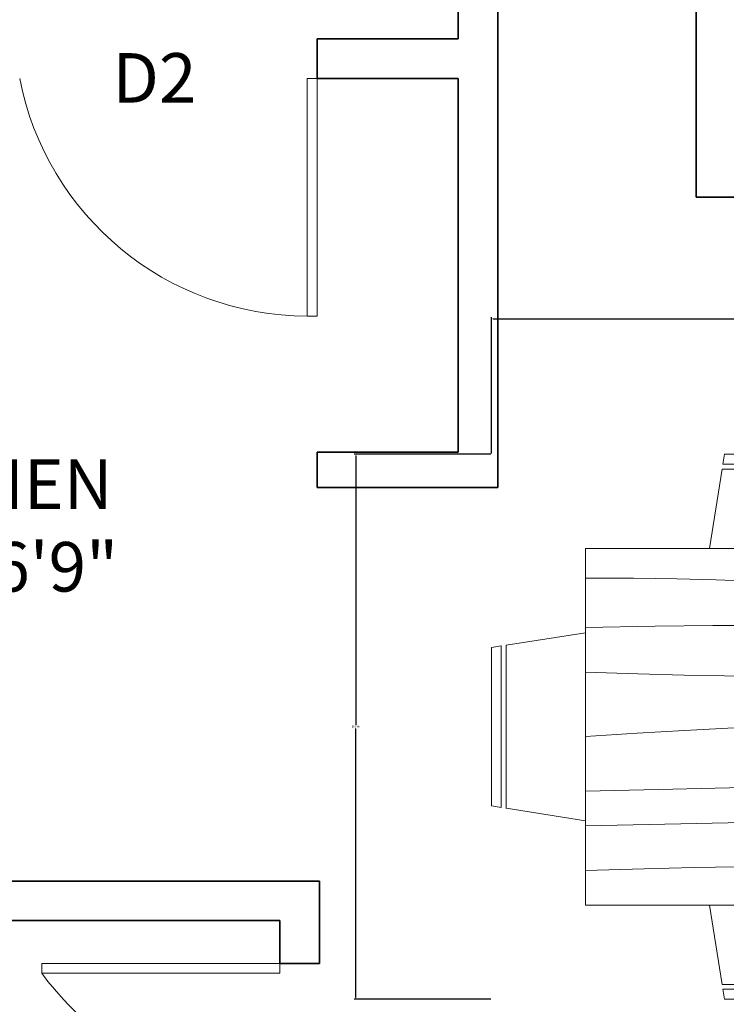
# Model space of a CAD drawing. Units: inches. Extents: x -86 to 2463, y -1058 to 68.
# Tile 14 of 17: x 77 to 148, y -114 to -14. Entities that reach past the tile are written whole.
import ezdxf

# ---------------------------------------------------------------- set-up
doc = ezdxf.new("R2010")
doc.units = ezdxf.units.IN
doc.header["$MEASUREMENT"] = 0
for name, color, linetype, lineweight in [('A-ANNO-DIMS', 2, 'Continuous', 18), ('A-ANNO-TEXT', 7, 'Continuous', 18), ('A-AREA-IDEN', 7, 'Continuous', 18), ('A-DOOR', 3, 'Continuous', 18), ('A-FURN', 8, 'Continuous', 18), ('A-WALL', 7, 'Continuous', 35)]:
    doc.layers.add(name, color=color, linetype=linetype, lineweight=lineweight)
doc.styles.get("Standard").update_dxf_attribs({"font": 'arial.ttf'})
doc.dimstyles.get("Standard").update_dxf_attribs({"dimtxt": 0.18, "dimasz": 0.18, "dimexe": 0.18, "dimexo": 0.0625, "dimgap": 0.09, "dimtad": 0, "dimtih": 1, "dimtoh": 1, "dimdec": 4, "dimzin": 0, "dimdsep": 46, "dimtxsty": 'Standard', "dimcen": 0.09, "dimadec": 0, "dimazin": 0, "dimtfac": 1, "dimtdec": 4, "dimtofl": 0, "dimtmove": 0, "dimatfit": 3, "dimfxl": 1, "dimtolj": 1, "dimtzin": 0, "dimarcsym": 0})

# ---------------------------------------------------------------- blocks, each defined once
blk = doc.blocks.new('Dining Set - 36 x 72 in.')
for p, q in [((-22, 27.5), (-22.1562, 26.50042)), ((-22, 27.5), (-6, 27.5)), ((-5.8437, 26.49966), (-6, 27.5)), ((6, 27.5), (5.8438, 26.50042)), ((6, 27.5), (22, 27.5)), ((22.1563, 26.49966), (22, 27.5)), ((-22.2343, 26.00059), (-23.4847, 17.99762)), ((-22.2304, 26), (-5.7608, 26)), ((-5.8416, 26.5), (-22.1534, 26.5)), ((-4.5152, 17.99762), (-5.7655, 25.99926)), ((5.7657, 26.00059), (4.5153, 17.99762)), ((5.7696, 26), (22.2392, 26)), ((22.1584, 26.5), (5.8466, 26.5)), ((23.4848, 17.99762), (22.2345, 25.99926)), ((36, 18), (-36, 18)), ((-36, 18), (-36, -18)), ((36, -18), (36, 18)), ((-44.0006, 8.23428), (-35.9976, 9.48474)), ((44.0006, 8.23428), (35.9976, 9.48474)), ((-45.5, 8), (-44.5004, 8.15617)), ((-45.5, 8), (-45.5, -8)), ((-44.5, -8.15843), (-44.5, 8.15338)), ((-44, 8.23041), (-44, -8.23915)), ((44, 8.23041), (44, -8.23915)), ((44.5, -8.15843), (44.5, 8.15338)), ((45.5, 8), (44.5005, 8.15617)), ((45.5, 8), (45.5, -8)), ((-44.4997, -8.15631), (-45.5, -8)), ((-35.9976, -9.48476), (-43.9993, -8.2345)), ((35.9976, -9.48476), (43.9993, -8.2345)), ((44.4997, -8.15631), (45.5, -8)), ((-36, -18), (36, -18)), ((-22.2343, -26.0006), (-23.4847, -17.99762)), ((-4.5152, -17.99762), (-5.7655, -25.99928)), ((5.7657, -26.0006), (4.5153, -17.99762)), ((23.4848, -17.99762), (22.2345, -25.99928)), ((-22.2304, -26), (-5.7608, -26)), ((-22, -27.5), (-22.1562, -26.50044)), ((-5.8416, -26.5), (-22.1534, -26.5)), ((-5.8437, -26.49967), (-6, -27.5)), ((5.7696, -26), (22.2392, -26)), ((6, -27.5), (5.8438, -26.50044)), ((22.1584, -26.5), (5.8466, -26.5)), ((22.1563, -26.49967), (22, -27.5)), ((-22, -27.5), (-6, -27.5)), ((6, -27.5), (22, -27.5))]:
    blk.add_line(p, q)
for points in [[(-36, 15), (-31.1772, 14.97754), (-26.8079, 14.91406), (-22.8538, 14.81543), (-19.276, 14.6875), (-16.0362, 14.53613), (-13.0957, 14.36718), (-10.4159, 14.18652), (-7.9583, 14), (-5.6904, 13.81315), (-3.6035, 13.63021), (-1.6954, 13.45508), (0.0365, 13.29166), (1.5945, 13.14388), (2.9811, 13.01562), (4.1988, 12.9108), (5.25, 12.83333), (6.1393, 12.78613), (6.8802, 12.76823), (7.4883, 12.77767), (7.9792, 12.8125), (8.3685, 12.87077), (8.6719, 12.95052), (8.9049, 13.0498), (9.0833, 13.16666), (9.2205, 13.29899), (9.3216, 13.44401), (9.3895, 13.59879), (9.4271, 13.76041), (9.4373, 13.92594), (9.4232, 14.09245), (9.3875, 14.257), (9.3333, 14.41666), (9.2638, 14.56917), (9.1836, 14.71484), (9.0975, 14.85465), (9.0104, 14.98958), (8.9272, 15.1206), (8.8529, 15.2487), (8.7922, 15.37483), (8.75, 15.5), (8.7305, 15.62467), (8.7344, 15.74739), (8.7617, 15.86621), (8.8125, 15.97916), (8.8867, 16.08431), (8.9844, 16.17968), (9.1055, 16.26334), (9.25, 16.33333), (9.4189, 16.38802), (9.6172, 16.42708), (9.8506, 16.45052), (10.125, 16.45833), (10.4463, 16.45052), (10.8203, 16.42708), (11.2529, 16.38802), (11.75, 16.33333), (12.3184, 16.26318), (12.9694, 16.17838), (13.7151, 16.07991), (14.5677, 15.96875), (15.5395, 15.84586), (16.6426, 15.71224), (17.8893, 15.56884), (19.2917, 15.41666), (20.859, 15.25667), (22.5879, 15.08984), (24.4721, 14.91715), (26.5052, 14.73958), (28.6809, 14.5581), (30.9929, 14.3737), (33.4347, 14.18733), (36, 14)], [(-36, 10), (-28.9766, 10.14274), (-23.1725, 10.20442), (-18.4241, 10.19775), (-14.5677, 10.13541), (-11.4399, 10.03011), (-8.877, 9.89453), (-6.7154, 9.74137), (-4.7917, 9.58333), (-2.9698, 9.43082), (-1.2246, 9.28515), (0.4415, 9.14534), (2.026, 9.01041), (3.5266, 8.87939), (4.9408, 8.7513), (6.266, 8.62516), (7.5, 8.5), (8.6411, 8.37549), (9.6914, 8.2539), (10.6538, 8.13818), (11.5312, 8.03125), (12.3267, 7.93603), (13.043, 7.85547), (13.6831, 7.79248), (14.25, 7.75), (14.7471, 7.7303), (15.1797, 7.73307), (15.5537, 7.75732), (15.875, 7.80208), (16.1494, 7.86637), (16.3828, 7.94922), (16.5811, 8.04964), (16.75, 8.16666), (16.8944, 8.29915), (17.0143, 8.44531), (17.1089, 8.60319), (17.1771, 8.77083), (17.218, 8.94629), (17.2305, 9.1276), (17.2137, 9.31282), (17.1667, 9.5), (17.0895, 9.6875), (16.987, 9.875), (16.8649, 10.0625), (16.7292, 10.25), (16.5856, 10.4375), (16.4401, 10.625), (16.2985, 10.8125), (16.1667, 11), (16.05, 11.18733), (15.9518, 11.3737), (15.8752, 11.5581), (15.8229, 11.73958), (15.798, 11.91715), (15.8034, 12.08984), (15.842, 12.25667), (15.9167, 12.41666), (16.0295, 12.56836), (16.1784, 12.70833), (16.3605, 12.83268), (16.5729, 12.9375), (16.8127, 13.01888), (17.0768, 13.07291), (17.3625, 13.0957), (17.6667, 13.08333), (17.9894, 13.03312), (18.3418, 12.94726), (18.7382, 12.82918), (19.1927, 12.68229), (19.7195, 12.51001), (20.3327, 12.31575), (21.0465, 12.10294), (21.875, 11.875), (22.8357, 11.63354), (23.959, 11.37304), (25.2786, 11.08618), (26.8282, 10.76562), (28.6414, 10.40405), (30.752, 9.99414), (33.1936, 9.52856), (36, 9)], [(-36, 5.5), (-30.7157, 5.3348), (-26.069, 5.20963), (-21.9946, 5.11767), (-18.4271, 5.05208), (-15.3009, 5.00602), (-12.5508, 4.97265), (-10.1112, 4.94515), (-7.9167, 4.91666), (-5.909, 4.88167), (-4.0586, 4.83984), (-2.3429, 4.79215), (-0.7396, 4.73958), (0.7739, 4.6831), (2.22, 4.6237), (3.6213, 4.56233), (5, 4.5), (6.373, 4.43782), (7.7344, 4.3776), (9.0723, 4.32129), (10.375, 4.27083), (11.6309, 4.22819), (12.8281, 4.19531), (13.9551, 4.17415), (15, 4.16666), (15.954, 4.17448), (16.819, 4.19791), (17.6001, 4.23698), (18.3021, 4.29166), (18.9299, 4.36198), (19.4883, 4.44791), (19.9823, 4.54948), (20.4167, 4.66666), (20.7969, 4.79899), (21.1302, 4.94401), (21.4245, 5.09879), (21.6875, 5.26041), (21.9271, 5.42594), (22.1511, 5.59245), (22.3672, 5.757), (22.5834, 5.91666), (22.8065, 6.06868), (23.0404, 6.21093), (23.2879, 6.34147), (23.5521, 6.45833), (23.8358, 6.55957), (24.142, 6.64323), (24.4735, 6.70735), (24.8334, 6.75), (25.2235, 6.76969), (25.642, 6.76692), (26.0858, 6.74267), (26.5521, 6.69791), (27.0379, 6.63362), (27.5404, 6.55078), (28.0565, 6.45036), (28.5834, 6.33333), (29.1242, 6.19987), (29.7071, 6.04687), (30.3661, 5.87044), (31.1354, 5.66666), (32.0493, 5.43164), (33.142, 5.16146), (34.4475, 4.85221), (36, 4.5)], [(-36, -1), (-30.7915, -0.6591), (-26.0195, -0.38216), (-21.6519, -0.16284), (-17.6563, 0.00521), (-14.0005, 0.12833), (-10.6523, 0.21289), (-7.5796, 0.26522), (-4.75, 0.29166), (-2.134, 0.29793), (0.2878, 0.28711), (2.5317, 0.26163), (4.6146, 0.22396), (6.5529, 0.17651), (8.3633, 0.12174), (10.0623, 0.06209), (11.6667, 0), (13.1899, -0.06201), (14.6341, -0.1211), (15.9982, -0.17432), (17.2813, -0.21875), (18.4823, -0.25147), (19.6003, -0.26953), (20.6343, -0.27002), (21.5834, -0.25), (22.4481, -0.20768), (23.2357, -0.14584), (23.9549, -0.06836), (24.6146, 0.02083), (25.2235, 0.11784), (25.7904, 0.21875), (26.3241, 0.31966), (26.8334, 0.41666), (27.3265, 0.50618), (27.8099, 0.58593), (28.2894, 0.65397), (28.7709, 0.70833), (29.2601, 0.74707), (29.763, 0.76823), (30.2855, 0.76985), (30.8334, 0.75), (31.4088, 0.70784), (31.9994, 0.64713), (32.589, 0.57275), (33.1615, 0.48958), (33.7008, 0.4025), (34.1908, 0.3164), (34.6153, 0.23616), (34.9584, 0.16666), (35.2099, 0.11165), (35.3848, 0.07031), (35.504, 0.04069), (35.5886, 0.02083), (35.6594, 0.00879), (35.7377, 0.0026), (35.8442, 0.00032), (36, 0)], [(-36, -6.5), (-27.1843, -6.31267), (-20.084, -6.1263), (-14.469, -5.9419), (-10.1094, -5.76042), (-6.7752, -5.58285), (-4.2363, -5.41016), (-2.2629, -5.24333), (-0.625, -5.08334), (0.8708, -4.93099), (2.2715, -4.78646), (3.5872, -4.64974), (4.8281, -4.52084), (6.0046, -4.39974), (7.127, -4.28646), (8.2053, -4.18099), (9.25, -4.08334), (10.2705, -3.99382), (11.2734, -3.91407), (12.2647, -3.84603), (13.25, -3.79167), (14.2354, -3.75293), (15.2266, -3.73177), (16.2295, -3.73015), (17.25, -3.75), (18.2912, -3.79248), (19.3451, -3.85547), (20.4009, -3.93604), (21.4479, -4.03125), (22.4754, -4.13819), (23.4727, -4.25391), (24.4289, -4.37549), (25.3334, -4.5), (26.1785, -4.62492), (26.9694, -4.74935), (27.7145, -4.87281), (28.4219, -4.99479), (29.1, -5.11483), (29.7572, -5.23242), (30.4016, -5.34709), (31.0417, -5.45834), (31.6837, -5.56437), (32.3262, -5.65821), (32.9658, -5.73153), (33.599, -5.77604), (34.2224, -5.78345), (34.8327, -5.74545), (35.4264, -5.65373), (36, -5.5)], [(-36, -10), (-26.4022, -9.81299), (-18.4675, -9.62891), (-11.9839, -9.45069), (-6.7396, -9.28125), (-2.5226, -9.12354), (0.8789, -8.98047), (3.6769, -8.85498), (6.0833, -8.75), (8.2767, -8.66765), (10.3021, -8.60677), (12.1712, -8.56543), (13.8958, -8.54167), (15.4876, -8.53353), (16.9583, -8.53907), (18.3197, -8.55632), (19.5834, -8.58334), (20.7616, -8.61841), (21.8685, -8.66081), (22.9188, -8.71004), (23.9271, -8.76563), (24.9081, -8.82707), (25.8763, -8.89388), (26.8465, -8.96558), (27.8334, -9.04167), (28.8474, -9.12118), (29.8828, -9.20117), (30.93, -9.27824), (31.9792, -9.34896), (33.0205, -9.40991), (34.0443, -9.45768), (35.0407, -9.48885), (36, -9.5)], [(-36, -14.5), (-30.0881, -14.33513), (-25.0332, -14.21224), (-20.7312, -14.12647), (-17.0781, -14.07292), (-13.97, -14.04671), (-11.3027, -14.04297), (-8.9724, -14.05681), (-6.875, -14.08334), (-4.9224, -14.11833), (-3.0905, -14.16016), (-1.3709, -14.20785), (0.2448, -14.26042), (1.7647, -14.3169), (3.1973, -14.3763), (4.5507, -14.43767), (5.8333, -14.5), (7.0554, -14.5621), (8.235, -14.62175), (9.3922, -14.67652), (10.5469, -14.72396), (11.7192, -14.76164), (12.929, -14.78711), (14.1965, -14.79794), (15.5417, -14.79167), (16.9933, -14.76424), (18.6152, -14.70508), (20.4804, -14.60197), (22.6615, -14.44271), (25.2312, -14.21509), (28.2624, -13.9069), (31.8277, -13.50594), (36, -13)]]:
    blk.add_lwpolyline(points)
blk = doc.blocks.new('DOOR-LEAF-24IN')
for p, q in [((0, 0), (0, 24)), ((0, 24), (1, 24)), ((1, 24), (1, 0)), ((1, 0), (0, 0))]:
    blk.add_line(p, q)
blk = doc.blocks.new('*D28')
at = {"layer": 'A-ANNO-DIMS', "color": 0, "lineweight": -2, "transparency": 16777216}
for p, q in [((124.097, -57.969), (124.097, -44.201)), ((124.277, -44.381), (168.319, -44.381)), ((214.917, -44.381), (170.875, -44.381)), ((215.097, -57.969), (215.097, -44.201))]:
    blk.add_line(p, q, dxfattribs=at)
at = {"layer": 'A-ANNO-DIMS', "color": 0, "transparency": 16777216}
for points in [[(124.277, -44.351), (124.277, -44.411), (124.097, -44.381)], [(214.917, -44.351), (214.917, -44.411), (215.097, -44.381)]]:
    blk.add_solid(points, dxfattribs=at)
at = {"layer": 'Defpoints', "color": 0, "transparency": 16777216}
for p in [(215.097, -44.381), (124.097, -58.031), (215.097, -58.031)]:
    blk.add_point(p, dxfattribs=at)
at = {"layer": 'A-ANNO-DIMS', "color": 0, "transparency": 16777216, "insert": (169.597, -44.381), "char_height": 0.18, "attachment_point": 5}
blk.add_mtext('\\A1;DINING SET 91 TYP.', dxfattribs=at)
blk = doc.blocks.new('*D29')
at = {"layer": 'A-ANNO-DIMS', "color": 0, "lineweight": -2, "transparency": 16777216}
for p, q in [((124.034, -58.031), (110.267, -58.031)), ((110.447, -58.211), (110.447, -85.349)), ((110.447, -112.851), (110.447, -85.713)), ((124.034, -113.031), (110.267, -113.031))]:
    blk.add_line(p, q, dxfattribs=at)
at = {"layer": 'A-ANNO-DIMS', "color": 0, "transparency": 16777216}
for points in [[(110.417, -58.211), (110.477, -58.211), (110.447, -58.031)], [(110.417, -112.851), (110.477, -112.851), (110.447, -113.031)]]:
    blk.add_solid(points, dxfattribs=at)
at = {"layer": 'Defpoints', "color": 0, "transparency": 16777216}
for p in [(110.447, -58.031), (124.097, -58.031), (124.097, -113.031)]:
    blk.add_point(p, dxfattribs=at)
at = {"layer": 'A-ANNO-DIMS', "color": 0, "transparency": 16777216, "insert": (110.447, -85.531), "char_height": 0.18, "attachment_point": 5}
blk.add_mtext('\\A1;55 TYP.', dxfattribs=at)

msp = doc.modelspace()

# ---------------------------------------------------------------- linework, layer by layer
at = {"layer": 'A-DOOR'}
for centre, radius, start, end in [((105.635, -14.459), 29.645, 190.97719, 269.80143), ((104.302, -91.48), 31.795, 216.55167, 274.43502)]:
    msp.add_arc(centre, radius, start, end, dxfattribs=at)
at = {"layer": 'A-WALL'}
for p, q in [((120.761, 19.896), (120.761, -16.104)), ((124.761, 19.896), (124.761, -61.399)), ((144.761, -32.104), (144.761, 19.896)), ((120.761, -16.104), (106.532, -16.104)), ((106.532, -16.104), (106.532, -20.104)), ((120.761, -20.104), (106.532, -20.104)), ((120.761, -20.104), (120.761, -57.827)), ((144.761, -32.104), (220.761, -32.104)), ((120.761, -57.827), (106.532, -57.827)), ((106.532, -57.827), (106.532, -61.399)), ((106.532, -61.399), (120.761, -61.399)), ((120.761, -61.399), (124.761, -61.399)), ((106.761, -101.104), (24.761, -101.104)), ((106.761, -105.104), (106.761, -101.104)), ((102.761, -105.104), (24.761, -105.104)), ((102.761, -105.104), (102.761, -109.415)), ((106.761, -105.104), (106.761, -109.415)), ((102.761, -109.415), (106.761, -109.415))]:
    msp.add_line(p, q, dxfattribs=at)

# ---------------------------------------------------------------- block references
at = {"layer": 'A-DOOR'}
msp.add_blockref('DOOR-LEAF-24IN', (105.532, -44.104), dxfattribs=at)
at = {"layer": 'A-DOOR', "rotation": 90}
msp.add_blockref('DOOR-LEAF-24IN', (102.761, -110.415), dxfattribs=at)
at = {"layer": 'A-FURN'}
msp.add_blockref('Dining Set - 36 x 72 in.', (169.597, -85.531), dxfattribs=at)

# ---------------------------------------------------------------- texts
at = {"layer": 'A-ANNO-TEXT', "insert": (85.879, -17.557), "char_height": 5, "attachment_point": 1}
msp.add_mtext_dynamic_manual_height_columns('D2', width=8.24973, gutter_width=25, heights=[0], dxfattribs=at)
at = {"layer": 'A-AREA-IDEN', "insert": (57.148, -58.557), "char_height": 5, "attachment_point": 1}
msp.add_mtext_dynamic_manual_height_columns('KITCHEN\\P8\'0"X6\'9"', width=26.29818, gutter_width=25, heights=[0], dxfattribs=at)

# ---------------------------------------------------------------- dimensions: what is measured, and where the dimension line sits
at = {"layer": 'A-ANNO-DIMS'}
dim = msp.add_linear_dim(base=(215.097, -44.381), p1=(124.097, -58.031), p2=(215.097, -58.031), text='DINING SET <> TYP.', dimstyle='Standard', override={"dimdec": 0, "dimlfac": 1, "dimrnd": 0, "dimzin": 0, "dimdsep": 46, "dimlunit": 2}, dxfattribs=at)
dim.commit()
dim.dimension.update_dxf_attribs({"geometry": '*D28', "text_midpoint": (169.597, -44.381)})
dim = msp.add_linear_dim(base=(110.447, -58.031), p1=(124.097, -113.031), p2=(124.097, -58.031), angle=90, text='<> TYP.', dimstyle='Standard', override={"dimdec": 0, "dimlfac": 1, "dimrnd": 0, "dimzin": 0, "dimdsep": 46, "dimlunit": 2}, dxfattribs=at)
dim.commit()
dim.dimension.update_dxf_attribs({"geometry": '*D29', "text_midpoint": (110.447, -85.531)})

doc.saveas('drawing.dxf')
